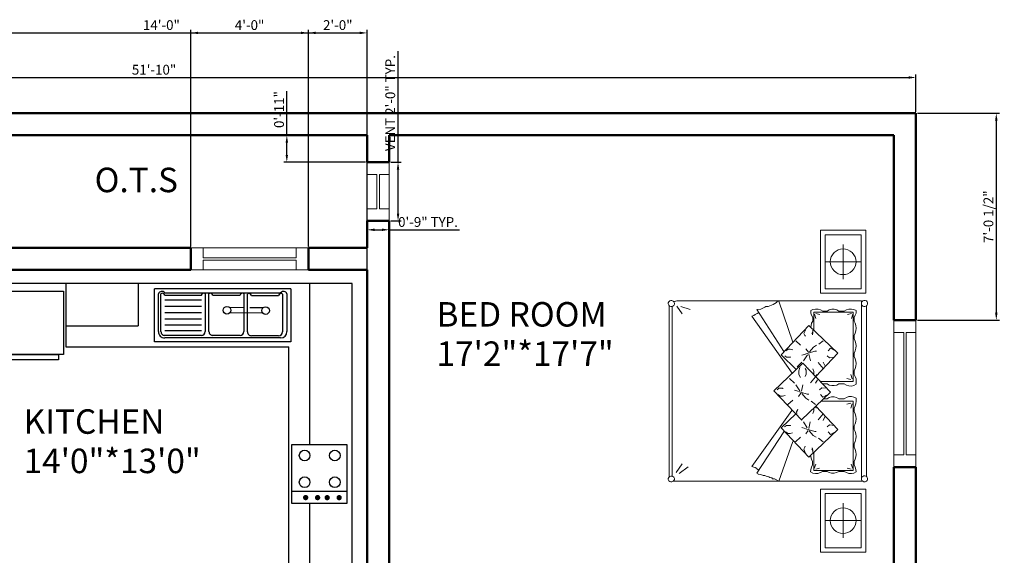
# Model space of a CAD drawing. Units: inches. Extents: x 2201 to 2875, y 1361 to 2074.
# Tile 4 of 4: x 2474 to 2875, y 1855 to 2074. Entities that reach past the tile are written whole.
import ezdxf

# ---------------------------------------------------------------- set-up
doc = ezdxf.new("R2010")
doc.units = ezdxf.units.IN
for name, color, linetype, lineweight in [('A-ANNO-DIMS', 2, 'Continuous', 18), ('A-AREA-IDEN', 7, 'Continuous', 25), ('A-FLOR-FIXT', 9, 'Continuous', 18), ('furniture', 8, 'Continuous', 18), ('ventilator', 3, 'Continuous', 18), ('walls', 6, 'Continuous', 50), ('windows', 4, 'Continuous', 18)]:
    doc.layers.add(name, color=color, linetype=linetype, lineweight=lineweight)
doc.layers.add('TEFRIŞ', color=11, linetype='Continuous')
doc.styles.get("Standard").update_dxf_attribs({"font": 'arial.ttf'})
doc.dimstyles.new('ISO-25', dxfattribs={"dimtxt": 4, "dimasz": 3, "dimexe": 1.25, "dimexo": 0.625, "dimtad": 1, "dimlunit": 3, "dimtxsty": 'Standard', "dimcen": 2.5, "dimadec": 0, "dimazin": 0, "dimtfac": 1, "dimtmove": 0, "dimatfit": 3, "dimfxl": 1, "dimarcsym": 0})

# ---------------------------------------------------------------- blocks, each defined once
blk = doc.blocks.new('d-bed-3')
at = {"color": 0, "linetype": 'ByBlock'}
for p, q in [((0, 0), (0, -0.5)), ((0.7, 0), (0, 0)), ((0.7, -0.5), (0.7, 0)), ((0.782, -0.005), (0.786, 0.008)), ((0.782, -0.005), (0.786, 0.008)), ((0.786, 0.008), (0.797, 0.017)), ((0.786, 0.008), (0.797, 0.017)), ((0.797, 0.017), (0.808, 0.021)), ((0.797, 0.017), (0.808, 0.021)), ((0.808, 0.021), (0.821, 0.021)), ((0.808, 0.021), (0.821, 0.021)), ((0.821, 0.021), (0.835, 0.014)), ((0.821, 0.021), (0.835, 0.014)), ((0.835, 0.014), (0.841, 0.008)), ((0.835, 0.014), (0.843, 0.006)), ((0.839, 0.008), (2.73, 0.008)), ((0.841, 0.008), (2.73, 0.008)), ((0.843, 0.006), (0.848, -0.008)), ((2.723, -0.008), (2.728, 0.006)), ((2.728, 0.006), (2.736, 0.014)), ((2.73, 0.008), (2.736, 0.014)), ((2.736, 0.014), (2.751, 0.021)), ((2.736, 0.014), (2.751, 0.021)), ((2.751, 0.021), (2.764, 0.021)), ((2.751, 0.021), (2.764, 0.021)), ((2.764, 0.021), (2.775, 0.017)), ((2.764, 0.021), (2.775, 0.017)), ((2.775, 0.017), (2.786, 0.008)), ((2.775, 0.017), (2.786, 0.008)), ((2.786, 0.008), (2.79, -0.005)), ((2.786, 0.008), (2.79, -0.005)), ((2.871, -0.5), (2.871, 0)), ((2.871, 0), (3.571, 0)), ((3.571, 0), (3.571, -0.5)), ((0.05, -0.05), (0.05, -0.45)), ((0.65, -0.05), (0.05, -0.05)), ((0.35, -0.058), (0.35, -0.442)), ((0.65, -0.45), (0.65, -0.05)), ((0.782, -0.019), (0.782, -0.005)), ((0.782, -0.019), (0.782, -0.005)), ((0.786, -0.03), (0.782, -0.019)), ((0.786, -0.03), (0.782, -0.019)), ((0.786, -2.094), (0.786, -0.03)), ((0.795, -0.041), (0.786, -0.03)), ((0.786, -0.032), (0.786, -2.094)), ((0.806, -0.045), (0.795, -0.041)), ((0.819, -0.045), (0.806, -0.045)), ((0.832, -0.041), (0.819, -0.045)), ((2.753, -0.045), (0.819, -0.045)), ((0.841, -0.032), (0.832, -0.041)), ((0.848, -0.021), (0.841, -0.032)), ((0.848, -0.008), (0.848, -0.021)), ((0.878, -0.132), (0.891, -0.106)), ((0.891, -0.106), (0.918, -0.108)), ((0.918, -0.108), (0.944, -0.115)), ((1.032, -0.117), (1.059, -0.108)), ((1.059, -0.108), (1.085, -0.106)), ((1.085, -0.106), (1.113, -0.11)), ((1.229, -0.117), (1.257, -0.108)), ((1.257, -0.108), (1.283, -0.106)), ((1.283, -0.106), (1.311, -0.11)), ((1.425, -0.117), (1.451, -0.108)), ((1.451, -0.108), (1.48, -0.106)), ((1.48, -0.106), (1.509, -0.11)), ((1.623, -0.115), (1.647, -0.108)), ((1.647, -0.108), (1.676, -0.106)), ((1.676, -0.106), (1.708, -0.106)), ((1.708, -0.106), (1.719, -0.132)), ((1.849, -0.13), (1.863, -0.106)), ((1.863, -0.106), (1.895, -0.106)), ((1.895, -0.106), (1.922, -0.106)), ((1.922, -0.106), (1.948, -0.115)), ((2.036, -0.115), (2.063, -0.108)), ((2.063, -0.108), (2.091, -0.106)), ((2.091, -0.106), (2.117, -0.108)), ((2.117, -0.108), (2.144, -0.115)), ((2.233, -0.115), (2.261, -0.108)), ((2.261, -0.108), (2.287, -0.106)), ((2.287, -0.106), (2.315, -0.108)), ((2.315, -0.108), (2.342, -0.115)), ((2.429, -0.115), (2.455, -0.108)), ((2.455, -0.108), (2.484, -0.106)), ((2.484, -0.106), (2.513, -0.108)), ((2.513, -0.108), (2.54, -0.115)), ((2.627, -0.115), (2.651, -0.106)), ((2.651, -0.106), (2.68, -0.106)), ((2.68, -0.106), (2.691, -0.13)), ((2.723, -0.021), (2.723, -0.008)), ((2.73, -0.032), (2.723, -0.021)), ((2.739, -0.041), (2.73, -0.032)), ((2.753, -0.045), (2.739, -0.041)), ((2.766, -0.045), (2.753, -0.045)), ((2.777, -0.041), (2.766, -0.045)), ((2.777, -0.041), (2.766, -0.045)), ((2.766, -0.045), (2.786, -0.045)), ((2.786, -0.045), (2.766, -0.045)), ((2.786, -0.03), (2.777, -0.041)), ((2.786, -0.03), (2.777, -0.041)), ((2.79, -0.019), (2.786, -0.03)), ((2.79, -0.019), (2.786, -0.03)), ((2.786, -2.094), (2.786, -0.045)), ((2.79, -0.005), (2.79, -0.019)), ((2.79, -0.005), (2.79, -0.019)), ((2.921, -0.45), (2.921, -0.05)), ((2.921, -0.05), (3.521, -0.05)), ((3.221, -0.058), (3.221, -0.442)), ((3.521, -0.05), (3.521, -0.45)), ((0.872, -0.159), (0.878, -0.132)), ((0.874, -0.187), (0.872, -0.159)), ((0.883, -0.213), (0.874, -0.187)), ((0.896, -0.237), (0.883, -0.213)), ((0.907, -0.575), (0.907, -0.139)), ((0.907, -0.139), (1.676, -0.139)), ((0.922, -0.161), (0.933, -0.204)), ((0.929, -0.143), (0.977, -0.161)), ((0.944, -0.115), (0.968, -0.128)), ((0.968, -0.128), (1.006, -0.128)), ((1.006, -0.128), (1.032, -0.117)), ((1.113, -0.11), (1.14, -0.117)), ((1.14, -0.117), (1.166, -0.128)), ((1.166, -0.128), (1.203, -0.128)), ((1.203, -0.128), (1.229, -0.117)), ((1.311, -0.11), (1.338, -0.117)), ((1.338, -0.117), (1.362, -0.128)), ((1.362, -0.128), (1.401, -0.128)), ((1.401, -0.128), (1.425, -0.117)), ((1.509, -0.11), (1.536, -0.117)), ((1.536, -0.117), (1.56, -0.128)), ((1.56, -0.128), (1.599, -0.128)), ((1.599, -0.128), (1.623, -0.115)), ((1.647, -0.15), (1.599, -0.166)), ((1.654, -0.166), (1.643, -0.209)), ((1.676, -0.139), (1.676, -0.494)), ((1.717, -0.213), (1.702, -0.237)), ((1.726, -0.187), (1.717, -0.213)), ((1.719, -0.132), (1.726, -0.159)), ((1.726, -0.159), (1.726, -0.187)), ((1.843, -0.159), (1.849, -0.13)), ((1.845, -0.187), (1.843, -0.159)), ((1.854, -0.213), (1.845, -0.187)), ((1.867, -0.237), (1.854, -0.213)), ((2.662, -0.137), (1.893, -0.137)), ((1.893, -0.137), (1.893, -0.505)), ((1.915, -0.166), (1.926, -0.209)), ((1.922, -0.148), (1.97, -0.166)), ((1.948, -0.115), (1.972, -0.128)), ((1.972, -0.128), (2.01, -0.128)), ((2.01, -0.128), (2.036, -0.115)), ((2.144, -0.115), (2.17, -0.128)), ((2.17, -0.128), (2.207, -0.128)), ((2.207, -0.128), (2.233, -0.115)), ((2.342, -0.115), (2.366, -0.128)), ((2.366, -0.128), (2.405, -0.128)), ((2.405, -0.128), (2.429, -0.115)), ((2.54, -0.115), (2.564, -0.128)), ((2.564, -0.128), (2.603, -0.128)), ((2.64, -0.143), (2.592, -0.159)), ((2.603, -0.128), (2.627, -0.115)), ((2.647, -0.159), (2.636, -0.202)), ((2.662, -0.575), (2.662, -0.137)), ((2.688, -0.213), (2.673, -0.237)), ((2.697, -0.187), (2.688, -0.213)), ((2.691, -0.13), (2.697, -0.159)), ((2.697, -0.159), (2.697, -0.187)), ((0.158, -0.25), (0.542, -0.25)), ((0.876, -0.349), (0.883, -0.324)), ((0.883, -0.324), (0.896, -0.299)), ((0.896, -0.299), (0.896, -0.237)), ((1.054, -0.629), (1.362, -0.308)), ((1.362, -0.308), (1.619, -0.553)), ((1.702, -0.237), (1.702, -0.299)), ((1.702, -0.299), (1.717, -0.324)), ((1.717, -0.324), (1.724, -0.349)), ((1.847, -0.349), (1.854, -0.321)), ((1.854, -0.321), (1.867, -0.297)), ((1.867, -0.297), (1.867, -0.237)), ((2.207, -0.308), (1.948, -0.553)), ((2.515, -0.629), (2.207, -0.308)), ((2.673, -0.237), (2.673, -0.297)), ((2.673, -0.297), (2.688, -0.321)), ((2.688, -0.321), (2.695, -0.349)), ((3.414, -0.25), (3.029, -0.25)), ((0.876, -0.378), (0.876, -0.349)), ((0.883, -0.404), (0.876, -0.378)), ((0.896, -0.428), (0.883, -0.404)), ((0.896, -0.478), (0.896, -0.428)), ((1.329, -0.351), (1.307, -0.391)), ((1.307, -0.391), (1.335, -0.417)), ((1.412, -0.402), (1.39, -0.428)), ((1.405, -0.347), (1.412, -0.402)), ((1.467, -0.713), (1.775, -0.391)), ((1.717, -0.404), (1.702, -0.428)), ((1.702, -0.428), (1.702, -0.465)), ((1.724, -0.378), (1.717, -0.404)), ((1.742, -0.435), (1.719, -0.474)), ((1.724, -0.349), (1.724, -0.378)), ((1.775, -0.391), (2.098, -0.698)), ((1.819, -0.431), (1.823, -0.485)), ((1.847, -0.375), (1.847, -0.349)), ((1.854, -0.404), (1.847, -0.375)), ((1.867, -0.428), (1.854, -0.404)), ((1.867, -0.478), (1.867, -0.428)), ((2.163, -0.344), (2.157, -0.4)), ((2.157, -0.4), (2.179, -0.428)), ((2.263, -0.389), (2.233, -0.417)), ((2.241, -0.351), (2.263, -0.389)), ((2.688, -0.404), (2.673, -0.428)), ((2.673, -0.428), (2.673, -0.476)), ((2.695, -0.375), (2.688, -0.404)), ((2.695, -0.349), (2.695, -0.375)), ((0, -0.5), (0.7, -0.5)), ((0.05, -0.45), (0.65, -0.45)), ((0.872, -0.558), (0.874, -0.529)), ((0.874, -0.529), (0.883, -0.502)), ((0.883, -0.502), (0.896, -0.478)), ((0.922, -0.553), (0.933, -0.511)), ((1.225, -0.472), (1.263, -0.522)), ((1.501, -0.451), (1.46, -0.472)), ((1.533, -0.472), (1.467, -0.527)), ((1.719, -0.474), (1.749, -0.5)), ((1.823, -0.485), (1.801, -0.511)), ((1.911, -0.533), (1.874, -0.555)), ((2.036, -0.472), (2.102, -0.527)), ((2.069, -0.451), (2.109, -0.472)), ((2.344, -0.472), (2.307, -0.52)), ((2.647, -0.553), (2.636, -0.509)), ((2.673, -0.476), (2.688, -0.5)), ((2.688, -0.5), (2.697, -0.527)), ((2.697, -0.527), (2.697, -0.555)), ((3.571, -0.5), (2.871, -0.5)), ((3.521, -0.45), (2.921, -0.45)), ((0.878, -0.584), (0.872, -0.558)), ((0.891, -0.61), (0.878, -0.584)), ((0.918, -0.607), (0.891, -0.61)), ((1.109, -0.575), (0.907, -0.575)), ((0.944, -0.601), (0.918, -0.607)), ((0.929, -0.571), (0.977, -0.553)), ((0.968, -0.589), (0.944, -0.601)), ((1.006, -0.589), (0.968, -0.589)), ((1.032, -0.6), (1.006, -0.589)), ((1.059, -0.607), (1.032, -0.6)), ((1.379, -0.936), (1.054, -0.629)), ((1.076, -0.61), (1.059, -0.607)), ((1.105, -0.586), (1.127, -0.586)), ((1.127, -0.586), (1.148, -0.597)), ((1.148, -0.597), (1.131, -0.586)), ((1.131, -0.586), (1.159, -0.593)), ((1.296, -0.582), (1.274, -0.549)), ((1.346, -0.625), (1.296, -0.582)), ((1.314, -0.663), (1.351, -0.636)), ((1.34, -0.564), (1.34, -0.549)), ((1.357, -0.625), (1.34, -0.564)), ((1.368, -0.663), (1.357, -0.625)), ((1.373, -0.629), (1.445, -0.614)), ((1.379, -0.647), (1.445, -0.691)), ((1.566, -0.575), (1.538, -0.586)), ((1.597, -0.575), (1.566, -0.575)), ((1.599, -0.549), (1.614, -0.555)), ((1.638, -0.555), (1.676, -0.605)), ((1.708, -0.665), (1.687, -0.632)), ((1.753, -0.649), (1.753, -0.632)), ((1.771, -0.709), (1.753, -0.649)), ((1.944, -0.555), (1.878, -0.61)), ((1.97, -0.547), (1.95, -0.555)), ((1.968, -0.575), (2.004, -0.575)), ((2.004, -0.575), (2.032, -0.586)), ((2.039, -0.643), (2.043, -0.64)), ((2.196, -0.629), (2.124, -0.612)), ((2.19, -0.645), (2.124, -0.689)), ((2.19, -0.936), (2.515, -0.629)), ((2.201, -0.663), (2.212, -0.623)), ((2.212, -0.623), (2.229, -0.564)), ((2.256, -0.663), (2.218, -0.634)), ((2.222, -0.623), (2.274, -0.58)), ((2.229, -0.564), (2.229, -0.547)), ((2.274, -0.58), (2.296, -0.547)), ((2.438, -0.586), (2.409, -0.591)), ((2.442, -0.586), (2.42, -0.597)), ((2.42, -0.597), (2.438, -0.586)), ((2.464, -0.586), (2.442, -0.586)), ((2.46, -0.575), (2.662, -0.575)), ((2.513, -0.605), (2.496, -0.607)), ((2.54, -0.6), (2.513, -0.605)), ((2.564, -0.586), (2.54, -0.6)), ((2.603, -0.586), (2.564, -0.586)), ((2.64, -0.569), (2.592, -0.553)), ((2.627, -0.6), (2.603, -0.586)), ((2.651, -0.607), (2.627, -0.6)), ((2.68, -0.607), (2.651, -0.607)), ((2.691, -0.584), (2.68, -0.607)), ((2.697, -0.555), (2.691, -0.584)), ((1.105, -0.669), (1.142, -0.685)), ((1.142, -0.685), (1.164, -0.674)), ((1.164, -0.674), (1.175, -0.669)), ((1.225, -0.779), (1.274, -0.724)), ((1.373, -0.669), (1.384, -0.707)), ((1.467, -0.713), (1.46, -0.707)), ((1.79, -1.019), (1.467, -0.713)), ((1.555, -0.767), (1.54, -0.763)), ((1.555, -0.767), (1.577, -0.756)), ((1.577, -0.756), (1.588, -0.752)), ((1.76, -0.709), (1.708, -0.665)), ((1.726, -0.745), (1.764, -0.72)), ((1.782, -0.745), (1.771, -0.709)), ((1.786, -0.713), (1.856, -0.698)), ((1.786, -0.752), (1.797, -0.79)), ((2.098, -0.698), (1.79, -1.019)), ((1.79, -0.731), (1.856, -0.774)), ((1.972, -0.741), (1.939, -0.724)), ((1.976, -0.66), (1.95, -0.671)), ((2.01, -0.741), (1.972, -0.741)), ((2.017, -0.66), (1.976, -0.66)), ((2.05, -0.731), (2.01, -0.741)), ((2.039, -0.671), (2.017, -0.66)), ((2.054, -0.761), (2.109, -0.707)), ((2.196, -0.667), (2.185, -0.707)), ((2.344, -0.776), (2.296, -0.722)), ((2.405, -0.674), (2.394, -0.667)), ((2.427, -0.685), (2.405, -0.674)), ((2.464, -0.667), (2.427, -0.685)), ((0.786, -0.961), (1.229, -0.807)), ((0.95, -1.261), (1.571, -0.818)), ((1.318, -0.838), (1.324, -0.812)), ((1.318, -0.86), (1.318, -0.838)), ((1.335, -0.888), (1.318, -0.86)), ((1.379, -0.936), (1.536, -0.776)), ((1.405, -0.834), (1.401, -0.834)), ((1.405, -0.877), (1.405, -0.834)), ((1.638, -0.862), (1.687, -0.807)), ((1.928, -0.845), (1.874, -0.79)), ((2.618, -1.261), (1.985, -0.816)), ((2.19, -0.936), (2.028, -0.77)), ((2.163, -0.876), (2.163, -0.832)), ((2.163, -0.832), (2.168, -0.832)), ((2.233, -0.886), (2.252, -0.86)), ((2.252, -0.838), (2.245, -0.809)), ((2.252, -0.86), (2.252, -0.838)), ((2.783, -0.961), (2.328, -0.807)), ((0.813, -1.012), (0.786, -0.961)), ((0.878, -1.206), (1.335, -0.906)), ((1.39, -0.899), (1.405, -0.877)), ((1.73, -0.921), (1.738, -0.894)), ((1.73, -0.943), (1.73, -0.921)), ((1.749, -0.972), (1.73, -0.943)), ((1.801, -0.983), (1.819, -0.961)), ((1.819, -0.917), (1.812, -0.917)), ((1.819, -0.961), (1.819, -0.917)), ((2.179, -0.897), (2.163, -0.876)), ((2.691, -1.206), (2.225, -0.906)), ((2.783, -0.961), (2.779, -0.983)), ((0.813, -1.033), (0.813, -1.012)), ((0.824, -1.041), (0.813, -1.033)), ((0.83, -1.063), (0.824, -1.041)), ((0.835, -1.075), (0.83, -1.063)), ((0.845, -1.103), (0.835, -1.075)), ((2.746, -1.026), (2.723, -1.081)), ((2.723, -1.081), (2.723, -1.108)), ((2.768, -0.989), (2.746, -1.026)), ((2.779, -0.983), (2.768, -0.989)), ((0.852, -1.119), (0.845, -1.103)), ((0.852, -1.136), (0.852, -1.119)), ((0.863, -1.162), (0.852, -1.136)), ((0.867, -1.19), (0.863, -1.162)), ((0.874, -1.195), (0.867, -1.19)), ((0.878, -1.206), (0.874, -1.195)), ((0.922, -1.202), (0.911, -1.184)), ((2.658, -1.184), (2.647, -1.202)), ((2.695, -1.162), (2.691, -1.206)), ((2.712, -1.125), (2.695, -1.162)), ((2.717, -1.119), (2.712, -1.125)), ((2.723, -1.108), (2.717, -1.119)), ((0.929, -1.206), (0.922, -1.202)), ((0.94, -1.224), (0.929, -1.206)), ((0.944, -1.239), (0.94, -1.224)), ((0.95, -1.261), (0.944, -1.239)), ((2.625, -1.239), (2.618, -1.261)), ((2.636, -1.224), (2.625, -1.239)), ((2.647, -1.202), (2.636, -1.224)), ((2.723, -2.05), (2.691, -1.947)), ((0.874, -2.067), (0.946, -1.969)), ((0.885, -2.1), (0.979, -2.034)), ((2.73, -2.094), (2.642, -2.034)), ((0.78, -2.148), (0.786, -2.135)), ((0.78, -2.148), (0.786, -2.135)), ((0.78, -2.159), (0.78, -2.148)), ((0.78, -2.148), (0.78, -2.159)), ((0.784, -2.172), (0.78, -2.159)), ((0.784, -2.172), (0.78, -2.159)), ((0.793, -2.181), (0.784, -2.172)), ((0.793, -2.181), (0.784, -2.172)), ((0.789, -2.132), (0.786, -2.094)), ((0.786, -2.094), (0.789, -2.13)), ((0.786, -2.135), (0.795, -2.126)), ((0.786, -2.135), (0.789, -2.132)), ((0.806, -2.188), (0.793, -2.181)), ((0.806, -2.188), (0.793, -2.181)), ((0.795, -2.126), (0.808, -2.121)), ((0.808, -2.121), (0.819, -2.121)), ((0.819, -2.121), (0.832, -2.128)), ((0.839, -2.174), (0.83, -2.183)), ((0.837, -2.177), (0.83, -2.183)), ((0.832, -2.128), (0.841, -2.137)), ((2.733, -2.177), (0.837, -2.177)), ((0.845, -2.161), (0.839, -2.174)), ((0.839, -2.177), (2.73, -2.177)), ((0.841, -2.137), (0.845, -2.15)), ((2.726, -2.144), (0.845, -2.144)), ((0.845, -2.15), (0.845, -2.161)), ((2.728, -2.137), (2.723, -2.15)), ((2.723, -2.15), (2.723, -2.161)), ((2.723, -2.161), (2.73, -2.174)), ((2.736, -2.128), (2.728, -2.137)), ((2.73, -2.174), (2.739, -2.183)), ((2.739, -2.183), (2.733, -2.177)), ((2.751, -2.121), (2.736, -2.128)), ((2.762, -2.121), (2.751, -2.121)), ((2.775, -2.126), (2.762, -2.121)), ((2.777, -2.181), (2.764, -2.188)), ((2.764, -2.188), (2.777, -2.181)), ((2.783, -2.135), (2.775, -2.126)), ((2.786, -2.172), (2.777, -2.181)), ((2.777, -2.181), (2.786, -2.172)), ((2.786, -2.094), (2.778, -2.13)), ((2.778, -2.13), (2.783, -2.135)), ((2.779, -2.128), (2.786, -2.094)), ((2.783, -2.135), (2.79, -2.148)), ((2.79, -2.148), (2.783, -2.135)), ((2.79, -2.159), (2.786, -2.172)), ((2.786, -2.172), (2.79, -2.159)), ((2.79, -2.148), (2.79, -2.159)), ((2.79, -2.159), (2.79, -2.148)), ((0.817, -2.188), (0.806, -2.188)), ((0.817, -2.188), (0.806, -2.188)), ((0.83, -2.183), (0.817, -2.188)), ((0.83, -2.183), (0.817, -2.188)), ((2.753, -2.188), (2.739, -2.183)), ((2.739, -2.183), (2.753, -2.188)), ((2.764, -2.188), (2.753, -2.188)), ((2.753, -2.188), (2.764, -2.188))]:
    blk.add_line(p, q, dxfattribs=at)
blk.add_ellipse((0.35, -0.25), major_axis=(-0.101, 0.101), ratio=1, dxfattribs=at)
at = {"color": 0, "linetype": 'ByBlock', "extrusion": (0, 0, -1)}
blk.add_ellipse((3.221, -0.25), major_axis=(0.101, 0.101), ratio=1, dxfattribs=at)
blk = doc.blocks.new('A$C008029BD')
at = {"layer": 'TEFRIŞ', "ltscale": 0.05}
for p, q in [((0, 0), (0, -3.55)), ((3.3699, 0), (0, 0)), ((3.3699, 0), (3.3699, -0.6)), ((1.5225, -0.4), (0, -0.4)), ((3.3699, -0.4), (2.0825, -0.4)), ((0.05, -0.5806), (0.05, -1.8694)), ((0.05, -0.5806), (0.55, -0.5806)), ((0.096, -0.6166), (0.454, -0.6166)), ((0.55, -0.5806), (0.55, -1.8694)), ((0.6, -2.71), (0.6, -0.6)), ((3.3699, -0.6), (0.6, -0.6)), ((0.086, -1.7734), (0.086, -0.6766)), ((0.0991, -0.6595), (0.4571, -0.6595)), ((0.1131, -0.954), (0.1131, -0.6955)), ((0.4931, -0.6955), (0.4931, -0.954)), ((0.514, -0.6766), (0.514, -1.7734)), ((0.2301, -0.8457), (0.2288, -0.9671)), ((0.2801, -0.8455), (0.2768, -1.1584)), ((0.096, -1.0242), (0.454, -1.0242)), ((0.4571, -0.99), (0.0991, -0.99)), ((0.2282, -1.0198), (0.2268, -1.1586)), ((0.11, -1.3187), (0.11, -1.0602)), ((0.49, -1.0602), (0.49, -1.3187)), ((0.454, -1.3547), (0.096, -1.3547)), ((0.096, -1.3912), (0.454, -1.3912)), ((0.11, -1.7734), (0.11, -1.4272)), ((0.1544, -1.7734), (0.1544, -1.4272)), ((0.2144, -1.7734), (0.2144, -1.4272)), ((0.2744, -1.7734), (0.2744, -1.4272)), ((0.3344, -1.7734), (0.3344, -1.4272)), ((0.3902, -1.7734), (0.3902, -1.4272)), ((0.4444, -1.7734), (0.4444, -1.4272)), ((0.49, -1.4272), (0.49, -1.7734)), ((0.454, -1.8094), (0.096, -1.8094)), ((0.454, -1.8334), (0.096, -1.8334)), ((0.55, -1.8694), (0.05, -1.8694)), ((0, -2.025), (0.4, -2.025)), ((0.4, -2.71), (0.4, -2.025)), ((0, -2.71), (0.6, -2.71)), ((0, -3.55), (0.65, -3.55))]:
    blk.add_line(p, q, dxfattribs=at)
at = {"layer": 'TEFRIŞ'}
blk.add_line((1.9688, -0.05), (1.9688, -0.5719), dxfattribs=at)
at = {"layer": 'TEFRIŞ', "ltscale": 0.05}
for points in [[(1.5225, -0.05), (2.0825, -0.05), (2.0825, -0.5719), (1.5225, -0.5719)], [(0.67, -2.73), (0.67, -3.53), (0.07, -3.53), (0.07, -2.73)], [(0.72, -2.78), (0.72, -3.48), (0.67, -3.48), (0.67, -2.78)]]:
    blk.add_lwpolyline(points, close=True, dxfattribs=at)
at = {"layer": 'TEFRIŞ', "const_width": 0.025}
for points in [[(2.0136, -0.1231, 1), (2.0386, -0.1231, 1)], [(2.0136, -0.2361, 1), (2.0386, -0.2361, 1)], [(2.0136, -0.3269, 1), (2.0386, -0.3269, 1)], [(2.0136, -0.4399, 1), (2.0386, -0.4399, 1)]]:
    blk.add_lwpolyline(points, format="xyb", close=True, dxfattribs=at)
at = {"layer": 'TEFRIŞ', "ltscale": 0.05}
for centre, radius in [((1.6277, -0.1636), 0.0505), ((1.6277, -0.4499), 0.0505), ((0.255, -0.8197), 0.036), ((0.2519, -1.1844), 0.036)]:
    blk.add_circle(centre, radius, dxfattribs=at)
at = {"layer": 'TEFRIŞ'}
for centre in [(1.8804, -0.1636), (1.8804, -0.4499)]:
    blk.add_circle(centre, 0.0505, dxfattribs=at)
at = {"layer": 'TEFRIŞ', "ltscale": 0.05}
for centre, radius, start, end in [((0.1083, -0.6495), 0.0351, 110.49764, 230.57771), ((0.454, -0.6766), 0.06, 0, 90), ((0.1177, -0.673), 0.023, 143.98534, 258.51568), ((0.4571, -0.6955), 0.036, 0, 90), ((0.1146, -1.0377), 0.023, 143.98534, 258.51568), ((0.1177, -0.9765), 0.023, 101.48432, 216.01466), ((0.454, -1.0602), 0.036, 0, 90), ((0.4571, -0.954), 0.036, 270, 0), ((0.1146, -1.3412), 0.023, 101.48432, 216.01466), ((0.1146, -1.4047), 0.023, 143.98534, 258.51568), ((0.454, -1.3187), 0.036, 270, 0), ((0.454, -1.4272), 0.036, 0, 90), ((0.1083, -1.8005), 0.0351, 129.42229, 249.50236), ((0.1146, -1.7959), 0.023, 101.48432, 216.01466), ((0.454, -1.7734), 0.06, 270, 0), ((0.454, -1.7734), 0.036, 270, 0)]:
    blk.add_arc(centre, radius, start, end, dxfattribs=at)
blk = doc.blocks.new('*D9')
at = {"layer": 'A-ANNO-DIMS', "color": 0, "lineweight": -2, "transparency": 16777216}
for p, q in [((2217.4, 2036.51), (2217.4, 2051.71)), ((2220.4, 2050.46), (2836.4, 2050.46)), ((2839.4, 2036.51), (2839.4, 2051.71))]:
    blk.add_line(p, q, dxfattribs=at)
at = {"layer": 'A-ANNO-DIMS', "color": 0, "transparency": 16777216}
for points in [[(2220.4, 2050.96), (2220.4, 2049.96), (2217.4, 2050.46)], [(2836.4, 2050.96), (2836.4, 2049.96), (2839.4, 2050.46)]]:
    blk.add_solid(points, dxfattribs=at)
at = {"layer": 'Defpoints', "color": 0, "transparency": 16777216}
for p in [(2839.4, 2050.46), (2217.4, 2035.88), (2839.4, 2035.88)]:
    blk.add_point(p, dxfattribs=at)
at = {"layer": 'A-ANNO-DIMS', "color": 0, "transparency": 16777216, "insert": (2528.4, 2053.13), "char_height": 4, "attachment_point": 5}
blk.add_mtext('51\'-10"', dxfattribs=at)
blk = doc.blocks.new('WIN-60IN')
for p, q in [((0, 9), (60, 9)), ((0, 0), (0, 9)), ((5, 5), (5, 9)), ((55, 9), (55, 5)), ((60, 9), (60, 0)), ((55, 5), (5, 5)), ((5, 0), (5, 4)), ((55, 4), (5, 4)), ((55, 4), (55, 0)), ((60, 0), (0, 0))]:
    blk.add_line(p, q)
blk = doc.blocks.new('VENT-24IN')
for p, q in [((0, 24), (0, 0)), ((9, 24), (0, 24)), ((9, 0), (9, 24)), ((4, 19), (0, 19)), ((4, 19), (4, 5)), ((9, 19), (5, 19)), ((5, 19), (5, 5)), ((0, 5), (4, 5)), ((5, 5), (9, 5)), ((0, 0), (9, 0))]:
    blk.add_line(p, q)
blk = doc.blocks.new('*D22')
at = {"layer": 'A-ANNO-DIMS', "color": 0, "lineweight": -2, "transparency": 16777216}
for p, q in [((2628, 2015.88), (2628, 2061.18)), ((2625.03, 2015.88), (2629.25, 2015.88)), ((2628, 1994.88), (2628, 2012.88)), ((2625.03, 1991.88), (2629.25, 1991.88))]:
    blk.add_line(p, q, dxfattribs=at)
at = {"layer": 'A-ANNO-DIMS', "color": 0, "transparency": 16777216}
for points in [[(2627.5, 2012.88), (2628.5, 2012.88), (2628, 2015.88)], [(2627.5, 1994.88), (2628.5, 1994.88), (2628, 1991.88)]]:
    blk.add_solid(points, dxfattribs=at)
at = {"layer": 'Defpoints', "color": 0, "transparency": 16777216}
for p in [(2624.4, 2015.88), (2628, 2015.88), (2624.4, 1991.88)]:
    blk.add_point(p, dxfattribs=at)
at = {"layer": 'A-ANNO-DIMS', "color": 0, "transparency": 16777216, "insert": (2625.34, 2040.03), "char_height": 4, "attachment_point": 5, "rotation": 90}
blk.add_mtext('VENT 2\'-0" TYP.', dxfattribs=at)
blk = doc.blocks.new('*D23')
at = {"layer": 'A-ANNO-DIMS', "color": 0, "lineweight": -2, "transparency": 16777216}
for p, q in [((2615.4, 1991.26), (2615.4, 1987.03)), ((2624.4, 1991.26), (2624.4, 1987.03)), ((2618.4, 1988.28), (2621.4, 1988.28)), ((2624.4, 1988.28), (2653.03, 1988.28))]:
    blk.add_line(p, q, dxfattribs=at)
at = {"layer": 'A-ANNO-DIMS', "color": 0, "transparency": 16777216}
for points in [[(2618.4, 1988.78), (2618.4, 1987.78), (2615.4, 1988.28)], [(2621.4, 1988.78), (2621.4, 1987.78), (2624.4, 1988.28)]]:
    blk.add_solid(points, dxfattribs=at)
at = {"layer": 'Defpoints', "color": 0, "transparency": 16777216}
for p in [(2615.4, 1991.88), (2624.4, 1991.88), (2624.4, 1988.28)]:
    blk.add_point(p, dxfattribs=at)
at = {"layer": 'A-ANNO-DIMS', "color": 0, "transparency": 16777216, "insert": (2640.22, 1990.95), "char_height": 4, "attachment_point": 5}
blk.add_mtext('0\'-9" TYP.', dxfattribs=at)
blk = doc.blocks.new('*D39')
at = {"layer": 'A-ANNO-DIMS', "color": 0, "lineweight": -2, "transparency": 16777216}
for p, q in [((2840.03, 2035.88), (2873.45, 2035.88)), ((2872.2, 2032.88), (2872.2, 1954.38)), ((2840.03, 1951.38), (2873.45, 1951.38))]:
    blk.add_line(p, q, dxfattribs=at)
at = {"layer": 'A-ANNO-DIMS', "color": 0, "transparency": 16777216}
for points in [[(2871.7, 2032.88), (2872.7, 2032.88), (2872.2, 2035.88)], [(2871.7, 1954.38), (2872.7, 1954.38), (2872.2, 1951.38)]]:
    blk.add_solid(points, dxfattribs=at)
at = {"layer": 'Defpoints', "color": 0, "transparency": 16777216}
for p in [(2839.4, 2035.88), (2839.4, 1951.38), (2872.2, 1951.38)]:
    blk.add_point(p, dxfattribs=at)
at = {"layer": 'A-ANNO-DIMS', "color": 0, "transparency": 16777216, "insert": (2869.51, 1993.63), "char_height": 4, "attachment_point": 5, "rotation": 90}
blk.add_mtext('7\'-0 1/2"', dxfattribs=at)
blk = doc.blocks.new('*D43')
at = {"layer": 'A-ANNO-DIMS', "color": 0, "lineweight": -2, "transparency": 16777216}
for p, q in [((2543.4, 1981.51), (2543.4, 2069.93)), ((2591.4, 1981.51), (2591.4, 2069.93)), ((2546.4, 2068.68), (2588.4, 2068.68))]:
    blk.add_line(p, q, dxfattribs=at)
at = {"layer": 'A-ANNO-DIMS', "color": 0, "transparency": 16777216}
for points in [[(2546.4, 2069.18), (2546.4, 2068.18), (2543.4, 2068.68)], [(2588.4, 2069.18), (2588.4, 2068.18), (2591.4, 2068.68)]]:
    blk.add_solid(points, dxfattribs=at)
at = {"layer": 'Defpoints', "color": 0, "transparency": 16777216}
for p in [(2591.4, 2068.68), (2543.4, 1980.88), (2591.4, 1980.88)]:
    blk.add_point(p, dxfattribs=at)
at = {"layer": 'A-ANNO-DIMS', "color": 0, "transparency": 16777216, "insert": (2567.4, 2071.35), "char_height": 4, "attachment_point": 5}
blk.add_mtext('4\'-0"', dxfattribs=at)
blk = doc.blocks.new('*D44')
at = {"layer": 'A-ANNO-DIMS', "color": 0, "lineweight": -2, "transparency": 16777216}
for p, q in [((2591.4, 1981.51), (2591.4, 2069.93)), ((2615.4, 1981.51), (2615.4, 2069.93)), ((2594.4, 2068.68), (2612.4, 2068.68))]:
    blk.add_line(p, q, dxfattribs=at)
at = {"layer": 'A-ANNO-DIMS', "color": 0, "transparency": 16777216}
for points in [[(2594.4, 2069.18), (2594.4, 2068.18), (2591.4, 2068.68)], [(2612.4, 2069.18), (2612.4, 2068.18), (2615.4, 2068.68)]]:
    blk.add_solid(points, dxfattribs=at)
at = {"layer": 'Defpoints', "color": 0, "transparency": 16777216}
for p in [(2615.4, 2068.68), (2591.4, 1980.88), (2615.4, 1980.88)]:
    blk.add_point(p, dxfattribs=at)
at = {"layer": 'A-ANNO-DIMS', "color": 0, "transparency": 16777216, "insert": (2603.4, 2071.35), "char_height": 4, "attachment_point": 5}
blk.add_mtext('2\'-0"', dxfattribs=at)
blk = doc.blocks.new('*D56')
at = {"layer": 'A-ANNO-DIMS', "color": 0, "lineweight": -2, "transparency": 16777216}
for p, q in [((2447.4, 1395.51), (2447.4, 2069.93)), ((2615.4, 1395.51), (2615.4, 2069.93)), ((2450.4, 2068.68), (2612.4, 2068.68))]:
    blk.add_line(p, q, dxfattribs=at)
at = {"layer": 'A-ANNO-DIMS', "color": 0, "transparency": 16777216}
for points in [[(2450.4, 2069.18), (2450.4, 2068.18), (2447.4, 2068.68)], [(2612.4, 2069.18), (2612.4, 2068.18), (2615.4, 2068.68)]]:
    blk.add_solid(points, dxfattribs=at)
at = {"layer": 'Defpoints', "color": 0, "transparency": 16777216}
for p in [(2615.4, 2068.68), (2447.4, 1394.88), (2615.4, 1394.88)]:
    blk.add_point(p, dxfattribs=at)
at = {"layer": 'A-ANNO-DIMS', "color": 0, "transparency": 16777216, "insert": (2531.4, 2071.35), "char_height": 4, "attachment_point": 5}
blk.add_mtext('14\'-0"', dxfattribs=at)
blk = doc.blocks.new('*D59')
at = {"layer": 'A-ANNO-DIMS', "color": 0, "lineweight": -2, "transparency": 16777216}
for p, q in [((2582.6, 2026.88), (2582.6, 2044.87)), ((2614.78, 2026.88), (2581.35, 2026.88)), ((2582.6, 2018.88), (2582.6, 2023.88)), ((2614.78, 2015.88), (2581.35, 2015.88))]:
    blk.add_line(p, q, dxfattribs=at)
at = {"layer": 'A-ANNO-DIMS', "color": 0, "transparency": 16777216}
for points in [[(2582.1, 2023.88), (2583.1, 2023.88), (2582.6, 2026.88)], [(2582.1, 2018.88), (2583.1, 2018.88), (2582.6, 2015.88)]]:
    blk.add_solid(points, dxfattribs=at)
at = {"layer": 'Defpoints', "color": 0, "transparency": 16777216}
for p in [(2582.6, 2026.88), (2615.4, 2026.88), (2615.4, 2015.88)]:
    blk.add_point(p, dxfattribs=at)
at = {"layer": 'A-ANNO-DIMS', "color": 0, "transparency": 16777216, "insert": (2579.94, 2037.38), "char_height": 4, "attachment_point": 5, "rotation": 90}
blk.add_mtext('0\'-11"', dxfattribs=at)

msp = doc.modelspace()

# ---------------------------------------------------------------- linework, layer by layer
at = {"layer": 'walls'}
for p, q in [((2217.403, 2035.883), (2839.403, 2035.883)), ((2839.403, 2035.883), (2839.403, 1951.383)), ((2447.403, 2026.883), (2615.403, 2026.883)), ((2615.403, 2026.883), (2615.403, 2015.883)), ((2624.403, 2026.883), (2624.403, 2015.883)), ((2624.403, 2026.883), (2830.403, 2026.883)), ((2830.403, 2026.883), (2830.403, 1951.383)), ((2624.403, 2015.883), (2615.403, 2015.883)), ((2624.403, 1991.883), (2615.403, 1991.883)), ((2615.403, 1991.883), (2615.403, 1980.883)), ((2624.403, 1991.883), (2624.403, 1815.883)), ((2447.403, 1980.883), (2543.403, 1980.883)), ((2543.403, 1980.883), (2543.403, 1971.883)), ((2591.403, 1980.883), (2591.403, 1971.883)), ((2591.403, 1980.883), (2615.403, 1980.883)), ((2447.403, 1971.883), (2543.403, 1971.883)), ((2591.403, 1971.883), (2615.403, 1971.883)), ((2615.403, 1971.883), (2615.403, 1815.883)), ((2830.403, 1951.383), (2839.403, 1951.383)), ((2830.403, 1891.383), (2830.403, 1815.883)), ((2830.403, 1891.383), (2839.403, 1891.383)), ((2839.403, 1891.383), (2839.403, 1775.383))]:
    msp.add_line(p, q, dxfattribs=at)
at = {"layer": 'windows'}
for p, q in [((2543.403, 1980.883), (2591.403, 1980.883)), ((2543.403, 1971.883), (2543.403, 1980.883)), ((2548.403, 1976.883), (2548.403, 1980.883)), ((2586.403, 1980.883), (2586.403, 1976.883)), ((2591.403, 1980.883), (2591.403, 1971.883)), ((2586.403, 1976.883), (2548.403, 1976.883)), ((2548.403, 1971.883), (2548.403, 1975.883)), ((2586.403, 1975.883), (2548.403, 1975.883)), ((2586.403, 1975.883), (2586.403, 1971.883)), ((2591.403, 1971.883), (2543.403, 1971.883))]:
    msp.add_line(p, q, dxfattribs=at)

# ---------------------------------------------------------------- block references
at = {"layer": 'A-FLOR-FIXT', "xscale": 43.13452976200671, "yscale": 43.13452976200671, "zscale": 43.13452976200671, "rotation": 270}
msp.add_blockref('A$C008029BD', (2609.265, 1966.296), dxfattribs=at)
at = {"layer": 'furniture', "xscale": -36.82314656981208, "yscale": 36.82314656981208, "zscale": 36.82314656981208, "rotation": 270}
msp.add_blockref('d-bed-3', (2818.887, 1856.615), dxfattribs=at)
at = {"layer": 'ventilator'}
msp.add_blockref('VENT-24IN', (2615.403, 1991.883), dxfattribs=at)
at = {"layer": 'windows', "rotation": 270.0000000000002}
msp.add_blockref('WIN-60IN', (2830.403, 1951.382), dxfattribs=at)

# ---------------------------------------------------------------- texts
at = {"layer": 'A-AREA-IDEN'}
for s, p in [('O.T.S', (2504.15, 2003.63)), ('BED ROOM', (2643.708, 1948.757)), ('17\'2"*17\'7"', (2643.708, 1932.693)), ('KITCHEN', (2475.146, 1904.968)), ('14\'0"*13\'0"', (2475.146, 1888.903))]:
    msp.add_text(s, height=10, dxfattribs=at).set_placement(p)

# ---------------------------------------------------------------- dimensions: what is measured, and where the dimension line sits
at = {"layer": 'A-ANNO-DIMS'}
for base, p1, p2, override, picture, middle in [((2615.403, 2068.683), (2447.403, 1394.883), (2615.403, 1394.883), {"dimdec": 1, "dimlfac": 1, "dimrnd": 0, "dimzin": 1, "dimdsep": 46, "dimlunit": 4, "dimfrac": 2}, '*D56', (2531.403, 2071.35)), ((2591.403, 2068.683), (2543.403, 1980.883), (2591.403, 1980.883), {"dimdec": 1, "dimlfac": 1, "dimrnd": 0, "dimzin": 1, "dimdsep": 46, "dimlunit": 4, "dimfrac": 2}, '*D43', (2567.403, 2071.35)), ((2615.403, 2068.683), (2591.403, 1980.883), (2615.403, 1980.883), {"dimdec": 1, "dimlfac": 1, "dimrnd": 0, "dimzin": 1, "dimdsep": 46, "dimlunit": 4, "dimfrac": 2}, '*D44', (2603.403, 2071.35)), ((2839.403, 2050.464), (2217.403, 2035.883), (2839.403, 2035.883), {"dimclrd": 0, "dimclre": 0, "dimclrt": 0}, '*D9', (2528.403, 2053.131))]:
    dim = msp.add_linear_dim(base=base, p1=p1, p2=p2, dimstyle='ISO-25', override=override, dxfattribs=at)
    dim.commit()
    dim.dimension.update_dxf_attribs({"geometry": picture, "text_midpoint": middle})
dim = msp.add_linear_dim(base=(2628.003, 2015.883), p1=(2624.403, 1991.883), p2=(2624.403, 2015.883), angle=90, text='VENT <> TYP.', dimstyle='ISO-25', override={"dimdec": 1, "dimlfac": 1, "dimrnd": 0, "dimzin": 1, "dimdsep": 46, "dimlunit": 4, "dimfrac": 2}, dxfattribs=at)
dim.commit()
dim.dimension.update_dxf_attribs({"geometry": '*D22', "text_midpoint": (2625.335, 2040.03)})
for base, p1, p2, picture, middle in [((2582.603, 2026.883), (2615.403, 2015.883), (2615.403, 2026.883), '*D59', (2579.935, 2037.378)), ((2872.203, 1951.383), (2839.403, 2035.883), (2839.403, 1951.383), '*D39', (2869.51, 1993.633))]:
    dim = msp.add_linear_dim(base=base, p1=p1, p2=p2, angle=90, dimstyle='ISO-25', override={"dimdec": 1, "dimlfac": 1, "dimrnd": 0, "dimzin": 1, "dimdsep": 46, "dimlunit": 4, "dimfrac": 2}, dxfattribs=at)
    dim.commit()
    dim.dimension.update_dxf_attribs({"geometry": picture, "text_midpoint": middle})
dim = msp.add_linear_dim(base=(2624.403, 1988.283), p1=(2615.403, 1991.883), p2=(2624.403, 1991.883), text='<> TYP.', dimstyle='ISO-25', override={"dimdec": 1, "dimlfac": 1, "dimrnd": 0, "dimzin": 1, "dimdsep": 46, "dimlunit": 4, "dimfrac": 2}, dxfattribs=at)
dim.commit()
dim.dimension.update_dxf_attribs({"geometry": '*D23', "text_midpoint": (2640.219, 1990.95)})

doc.saveas('drawing.dxf')
